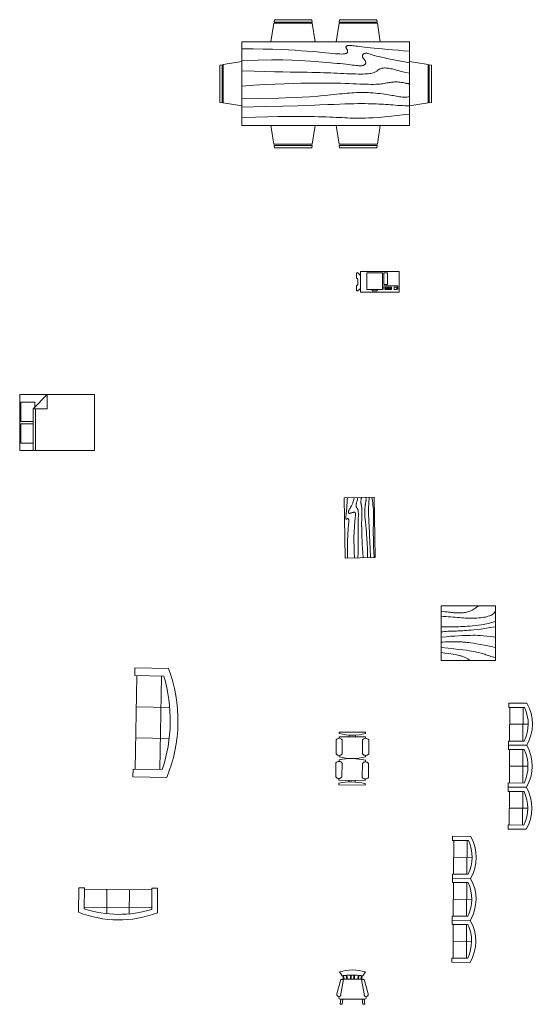
# Model space of a CAD drawing. Units: inches. Extents: x -1085 to 1941, y 1514 to 2348.
# Tile 5 of 9: x -255 to 142, y 1589 to 2348. Entities that reach past the tile are written whole.
import ezdxf

# ---------------------------------------------------------------- set-up
doc = ezdxf.new("R2010")
doc.units = ezdxf.units.IN
doc.layers.add('A-EQPM', color=9, linetype='Continuous', lineweight=18)
doc.layers.add('FOUNITR-URE', color=2, linetype='Continuous', lineweight=18)

# ---------------------------------------------------------------- blocks, each defined once
blk = doc.blocks.new('Bed - Queen')
for p, q in [((0, -80.00003), (0, 0)), ((0, 0), (59.99999, 0)), ((59.99999, 0), (59.99999, -80.00003)), ((7.99999, -1.2), (28.79998, -1.2)), ((7.99999, -14.4), (7.99999, -1.2)), ((28.79998, -1.2), (28.79998, -14.4)), ((31.19999, -1.2), (51.99999, -1.2)), ((31.19999, -14.4), (31.19999, -1.2)), ((51.99999, -1.2), (51.99999, -16.4)), ((0, -14.4), (44.8, -14.4)), ((44.8, -16.8), (0, -16.8)), ((59.99999, -29.6), (44.8, -14.4)), ((44.8, -14.4), (44.8, -29.6)), ((51.99999, -16.4), (46.79936, -16.4)), ((44.8, -29.6), (59.99999, -29.6)), ((59.99999, -80.00003), (0, -80.00003))]:
    blk.add_line(p, q)
blk = doc.blocks.new('Chair - Desk')
for p, q in [((-8.5, 0), (-8.5, -1)), ((-8.5, 0), (8.5, 0)), ((8.5, 0), (8.5, -1)), ((-10.5, -5), (-10.5, -14)), ((-8.5, -3), (-8.5, -4)), ((-8.5, -3), (8.5, -3)), ((-6.5, -14), (-6.5, -5)), ((-2, -3), (-2, -1.9355)), ((2, -1.9576), (2, -3)), ((6.5, -5), (6.5, -14)), ((8.5, -3), (8.5, -4)), ((10.5, -14), (10.5, -5)), ((-8.5, -15), (-8.5, -16)), ((8.5, -15), (8.5, -16))]:
    blk.add_line(p, q)
for centre, radius, start, end in [((-8.5, -6.5), 2.5, 36.8699, 143.1301), ((0, 34.625), 36.625, 256.5803, 283.4197), ((8.5, -6.5), 2.5, 36.8699, 143.1301), ((-8.5, -12.5), 2.5, 216.8699, 323.1301), ((0, 19.625), 36.625, 256.5803, 283.4197), ((8.5, -12.5), 2.5, 216.8699, 323.1301)]:
    blk.add_arc(centre, radius, start, end)
blk = doc.blocks.new('Sofa - Roundback Loveseat 5 ft.')
for p, q in [((-24, -33.99998), (-24, -11.46958)), ((-23.9998, -13.38178), (23.99986, -13.38178)), ((0, -32.44198), (0, -5.99998)), ((24.00004, -33.99998), (24.00004, -11.46958)), ((-24, -32.44198), (24.00004, -32.44198))]:
    blk.add_line(p, q)
for points in [[(-24, -33.99998), (-30, -33.99998), (-30, -7.99998)], [(30.00004, -7.99998), (30.00004, -33.99998), (24.00004, -33.99998)]]:
    blk.add_lwpolyline(points)
for centre, radius, start, end in [((0, -60.24998), 60.24998, 60.13715, 119.8628), ((0, -61.38438), 55.38444, 64.32083, 115.6792)]:
    blk.add_arc(centre, radius, start, end)
blk = doc.blocks.new('Table - Square Woodgrain 42 x 42 in.')
blk.add_line((0, -42), (42, -42))
for points in [[(0, -4), (1.704, -4.2172), (3.2358, -4.4188), (4.615, -4.604), (5.8615, -4.7721), (6.9951, -4.9224), (8.0357, -5.0541), (9.0031, -5.1667), (9.9171, -5.2594), (10.7951, -5.3316), (11.6445, -5.3836), (12.4702, -5.4157), (13.277, -5.4283), (14.0698, -5.4217), (14.8535, -5.3964), (15.6331, -5.3526), (16.4133, -5.2908), (17.1986, -5.2103), (17.9913, -5.1062), (18.793, -4.9727), (19.6056, -4.8038), (20.4307, -4.5937), (21.2701, -4.3365), (22.1256, -4.0262), (22.9989, -3.6571), (23.888, -3.2272), (24.7756, -2.7516), (25.6408, -2.2491), (26.4624, -1.7387), (27.2195, -1.2395), (27.891, -0.7703), (28.456, -0.3501), (28.8934, 0.002)], [(0, -42), (0, 0), (42, 0), (42, -42)], [(0, -8), (1.8203, -8.1001), (3.6741, -8.2149), (5.5411, -8.3408), (7.4011, -8.4741), (9.2339, -8.6112), (11.0193, -8.7484), (12.7371, -8.8821), (14.3671, -9.0086), (15.8954, -9.1246), (17.3337, -9.2278), (18.6997, -9.3159), (20.0116, -9.387), (21.2871, -9.4389), (22.5442, -9.4696), (23.8008, -9.477), (25.0749, -9.459), (26.3791, -9.4137), (27.7049, -9.3403), (29.0383, -9.2382), (30.3655, -9.1068), (31.6728, -8.9455), (32.9461, -8.7535), (34.1717, -8.5304), (35.3358, -8.2756), (36.4268, -7.9863), (37.443, -7.6521), (38.3849, -7.2603), (39.253, -6.7986), (40.048, -6.2542), (40.7705, -5.6147), (41.421, -4.8674), (42, -4)], [(42, -12), (39.1784, -12.8621), (36.4519, -13.5654), (33.8246, -14.1294), (31.3004, -14.5731), (28.8832, -14.9161), (26.577, -15.1775), (24.3858, -15.3768), (22.3136, -15.5332), (20.3622, -15.6632), (18.5254, -15.7718), (16.7947, -15.8612), (15.1618, -15.9338), (13.6183, -15.9916), (12.1558, -16.0369), (10.7659, -16.0718), (9.4403, -16.0987), (8.1703, -16.1191), (6.9461, -16.1325), (5.7577, -16.1377), (4.595, -16.1335), (3.4479, -16.1188), (2.3064, -16.0924), (1.1604, -16.0532), (0, -16)], [(42, -16), (37.6529, -16.7365), (33.8802, -17.329), (30.6179, -17.7961), (27.8015, -18.1561), (25.3668, -18.4275), (23.2497, -18.6288), (21.3859, -18.7785), (19.7111, -18.8949), (18.1693, -18.9939), (16.7375, -19.0795), (15.401, -19.1534), (14.1449, -19.217), (12.9544, -19.2717), (11.8148, -19.3191), (10.7113, -19.3606), (9.6291, -19.3976), (8.5534, -19.4323), (7.47, -19.4689), (6.3643, -19.5122), (5.222, -19.5672), (4.0288, -19.6386), (2.7703, -19.7313), (1.4321, -19.8501), (0, -20)], [(0, -24), (3.9243, -23.6805), (7.4766, -23.4138), (10.6891, -23.1954), (13.5943, -23.0205), (16.2247, -22.8847), (18.6125, -22.7832), (20.7903, -22.7116), (22.7903, -22.6651), (24.6563, -22.642), (26.4764, -22.6507), (28.35, -22.7024), (30.3766, -22.8084), (32.6555, -22.98), (35.2861, -23.2283), (38.3678, -23.5645), (42, -24)], [(42, -32), (37.392, -31.017), (33.4585, -30.2231), (30.1291, -29.5949), (27.3334, -29.109), (25.0009, -28.742), (23.0612, -28.4707), (21.4439, -28.2716), (20.0786, -28.1215), (18.8998, -28.0002), (17.8609, -27.9014), (16.9206, -27.8219), (16.0371, -27.7588), (15.1691, -27.709), (14.2748, -27.6693), (13.3128, -27.6368), (12.2415, -27.6083), (11.0295, -27.5824), (9.6867, -27.5643), (8.233, -27.5608), (6.6884, -27.5787), (5.0728, -27.6248), (3.4062, -27.7058), (1.7086, -27.8286), (0, -28)], [(0, -32), (5.4026, -32.5358), (9.9494, -33.019), (13.7424, -33.4553), (16.8834, -33.8505), (19.4743, -34.2106), (21.6171, -34.5413), (23.4136, -34.8486), (24.9657, -35.1382), (26.3614, -35.4156), (27.6332, -35.6841), (28.7995, -35.9467), (29.8788, -36.2064), (30.8897, -36.4661), (31.8507, -36.7288), (32.7802, -36.9973), (33.6968, -37.2747), (34.6175, -37.5635), (35.5531, -37.8651), (36.5128, -38.1805), (37.506, -38.5108), (38.5421, -38.8568), (39.6302, -39.2197), (40.7797, -39.6004), (42, -40)], [(0, -36), (3.0098, -36.2857), (5.5354, -36.5643), (7.6368, -36.8359), (9.374, -37.1009), (10.807, -37.3597), (11.9957, -37.6126), (13.0002, -37.8599), (13.8804, -38.102), (14.6874, -38.3393), (15.4365, -38.5729), (16.1338, -38.8041), (16.7858, -39.0341), (17.3987, -39.264), (17.9787, -39.4952), (18.5322, -39.7288), (19.0655, -39.9662), (19.5832, -40.2081), (20.0842, -40.4544), (20.5657, -40.7046), (21.0249, -40.9581), (21.459, -41.2144), (21.8653, -41.4731), (22.2409, -41.7335), (22.5831, -41.9951)]]:
    blk.add_lwpolyline(points)
blk = doc.blocks.new('Table - Rectangular Woodgrain 60 x 30 in.')
for p, q in [((0, 0), (0, -30)), ((60, 0), (0, 0)), ((60, -30), (60, 0)), ((0, -30), (60, -30))]:
    blk.add_line(p, q)
for points in [[(0, -2.4), (4.8155, -2.418), (9.0302, -2.4688), (12.709, -2.5477), (15.9167, -2.65), (18.7181, -2.7711), (21.1781, -2.9063), (23.3616, -3.0508), (25.3333, -3.2), (27.1477, -3.3495), (28.8172, -3.4958), (30.3437, -3.636), (31.7291, -3.7667), (32.9756, -3.8849), (34.0849, -3.9875), (35.059, -4.0714), (35.9, -4.1334), (36.6114, -4.1711), (37.2041, -4.1854), (37.6906, -4.1779), (38.0833, -4.15), (38.3948, -4.1034), (38.6375, -4.0396), (38.8239, -3.9602), (38.9666, -3.8667), (39.0764, -3.7608), (39.1573, -3.6448), (39.2116, -3.521), (39.2416, -3.3917), (39.2498, -3.2593), (39.2385, -3.1261), (39.21, -2.9944), (39.1666, -2.8667), (39.111, -2.7447), (39.0468, -2.6281), (38.978, -2.5163), (38.9083, -2.4083), (38.8418, -2.3035), (38.7823, -2.201), (38.7337, -2.1001), (38.7, -2), (38.6844, -1.9003), (38.6875, -1.8021), (38.7094, -1.707), (38.75, -1.6167), (38.8094, -1.5326), (38.8875, -1.4563), (38.9844, -1.3893), (39.1, -1.3333), (39.2351, -1.2896), (39.3937, -1.2583), (39.5804, -1.2396), (39.8, -1.2333), (40.057, -1.2396), (40.3562, -1.2583), (40.7023, -1.2896), (41.1, -1.3333), (41.5547, -1.3895), (42.0755, -1.4573), (42.6721, -1.5361), (43.3542, -1.625), (44.1316, -1.7233), (45.014, -1.8302), (46.0114, -1.9449), (47.1333, -2.0667), (48.3862, -2.1947), (49.7625, -2.3281), (51.2513, -2.4663), (52.8416, -2.6083), (54.5226, -2.7535), (56.2833, -2.9011), (58.1127, -3.0501), (60, -3.2)], [(0, -9.2), (6.5759, -9.0858), (11.9385, -9.0365), (16.2527, -9.0418), (19.6833, -9.0917), (22.3952, -9.1759), (24.5531, -9.2844), (26.322, -9.4069), (27.8666, -9.5333), (29.3241, -9.6553), (30.7203, -9.7719), (32.0532, -9.8837), (33.3208, -9.9917), (34.5213, -10.0965), (35.6526, -10.199), (36.7128, -10.2999), (37.7, -10.4), (38.6129, -10.4996), (39.4531, -10.5969), (40.223, -10.6895), (40.925, -10.775), (41.5613, -10.8512), (42.1344, -10.9156), (42.6465, -10.966), (43.1, -11), (43.4976, -11.0158), (43.8437, -11.0136), (44.143, -10.9942), (44.4, -10.9583), (44.6195, -10.9069), (44.8062, -10.8406), (44.9648, -10.7603), (45.1, -10.6667), (45.2155, -10.5598), (45.3114, -10.4365), (45.3871, -10.2929), (45.4416, -10.125), (45.4743, -9.929), (45.4844, -9.7011), (45.4709, -9.4371), (45.4333, -9.1333), (45.3716, -8.7883), (45.2896, -8.4104), (45.1919, -8.0107), (45.0833, -7.6), (44.9685, -7.1893), (44.8521, -6.7896), (44.7388, -6.4117), (44.6333, -6.0667), (44.54, -5.7628), (44.4614, -5.4979), (44.4001, -5.2675), (44.3583, -5.0667), (44.3384, -4.8909), (44.3427, -4.7354), (44.3736, -4.5956), (44.4333, -4.4667), (44.5236, -4.3453), (44.6427, -4.2333), (44.7884, -4.1339), (44.9583, -4.05), (45.1501, -3.9849), (45.3614, -3.9417), (45.59, -3.9234), (45.8333, -3.9333), (46.0915, -3.9749), (46.3734, -4.0531), (46.6906, -4.1736), (47.0542, -4.3417), (47.4756, -4.5629), (47.9661, -4.8427), (48.5372, -5.1866), (49.2, -5.6), (49.9676, -6.0844), (50.8594, -6.625), (51.8965, -7.2031), (53.1, -7.8), (54.491, -8.3969), (56.0906, -8.975), (57.9199, -9.5156), (60, -10)], [(0, -12.8), (5.1847, -12.9322), (9.6213, -13.0323), (13.3963, -13.1059), (16.5958, -13.1583), (19.3063, -13.1952), (21.614, -13.2219), (23.6054, -13.2439), (25.3666, -13.2667), (26.9728, -13.2947), (28.4531, -13.3281), (29.8256, -13.3663), (31.1083, -13.4083), (32.3191, -13.4535), (33.476, -13.501), (34.597, -13.5501), (35.7, -13.6), (36.7984, -13.6497), (37.8875, -13.6979), (38.9578, -13.743), (40, -13.7833), (41.0047, -13.8174), (41.9625, -13.8438), (42.864, -13.8607), (43.7, -13.8667), (44.4631, -13.8604), (45.1552, -13.8417), (45.7801, -13.8104), (46.3416, -13.7667), (46.8439, -13.7104), (47.2906, -13.6417), (47.6858, -13.5604), (48.0333, -13.4667), (48.3375, -13.3608), (48.6042, -13.2448), (48.8396, -13.121), (49.05, -12.9917), (49.2417, -12.8593), (49.4208, -12.7261), (49.5937, -12.5944), (49.7667, -12.4667), (49.9452, -12.3451), (50.1323, -12.2313), (50.3303, -12.1268), (50.5416, -12.0333), (50.7686, -11.9524), (51.0135, -11.8854), (51.2788, -11.8341), (51.5666, -11.8), (51.8785, -11.7843), (52.2116, -11.7865), (52.562, -11.8059), (52.926, -11.8417), (53.2998, -11.8931), (53.6795, -11.9594), (54.0614, -12.0397), (54.4416, -12.1333), (54.8223, -12.2401), (55.2293, -12.3625), (55.6942, -12.5037), (56.2489, -12.6667), (56.9251, -12.8547), (57.7545, -13.0708), (58.7689, -13.3182), (60, -13.6)], [(0, -18), (5.124, -17.7273), (9.6609, -17.5057), (13.6705, -17.3303), (17.2125, -17.1958), (20.3467, -17.0973), (23.1328, -17.0297), (25.6307, -16.9878), (27.9, -16.9667), (29.9928, -16.9617), (31.9302, -16.9703), (33.7254, -16.9907), (35.3917, -17.0208), (36.9423, -17.0588), (38.3906, -17.1026), (39.7499, -17.1503), (41.0333, -17.2), (42.2519, -17.2496), (43.4073, -17.2969), (44.4986, -17.3395), (45.525, -17.375), (46.4858, -17.4012), (47.3802, -17.4156), (48.2074, -17.416), (48.9667, -17.4), (49.6583, -17.3662), (50.2872, -17.3167), (50.8595, -17.2547), (51.3812, -17.1833), (51.8584, -17.1057), (52.2971, -17.025), (52.7034, -16.9443), (53.0833, -16.8667), (53.443, -16.7951), (53.789, -16.7313), (54.128, -16.6768), (54.4666, -16.6334), (54.8115, -16.6024), (55.1693, -16.5854), (55.5465, -16.5841), (55.95, -16.6), (56.3828, -16.6337), (56.8346, -16.6823), (57.2915, -16.7418), (57.7396, -16.8084), (58.165, -16.878), (58.5539, -16.9469), (58.8924, -17.0111), (59.1666, -17.0667), (59.3679, -17.1107), (59.5078, -17.1438), (59.6032, -17.1675), (59.6708, -17.1833), (59.7275, -17.193), (59.7901, -17.1979), (59.8753, -17.1998), (60, -17.2)], [(0, -22.4), (8.0098, -22.2501), (14.4094, -22.1011), (19.4168, -21.9535), (23.25, -21.8083), (26.1269, -21.6663), (28.2656, -21.5281), (29.884, -21.3947), (31.2, -21.2667), (32.3967, -21.1448), (33.5172, -21.0292), (34.5697, -20.9198), (35.5625, -20.8167), (36.5037, -20.7198), (37.4015, -20.6292), (38.2642, -20.5448), (39.1, -20.4667), (39.9164, -20.3951), (40.7187, -20.3313), (41.5117, -20.2768), (42.3, -20.2333), (43.0883, -20.2024), (43.8812, -20.1854), (44.6836, -20.1841), (45.5, -20.2), (46.3328, -20.234), (47.1747, -20.2844), (48.0163, -20.3488), (48.8479, -20.425), (49.66, -20.5106), (50.4429, -20.6031), (51.1872, -20.7004), (51.8833, -20.8), (52.5246, -20.8999), (53.1166, -20.9995), (53.6681, -21.0983), (54.1875, -21.1958), (54.6834, -21.2919), (55.1646, -21.3859), (55.6394, -21.4777), (56.1167, -21.5667), (56.6028, -21.6515), (57.0961, -21.7266), (57.5929, -21.7852), (58.0896, -21.8208), (58.5823, -21.8268), (59.0674, -21.7964), (59.5412, -21.723), (60, -21.6)], [(0, -25.2), (8.6355, -25.0504), (15.7026, -24.9031), (21.4049, -24.7606), (25.9458, -24.625), (29.529, -24.4988), (32.3578, -24.3844), (34.6359, -24.284), (36.5667, -24.2), (38.3213, -24.1341), (39.9417, -24.0854), (41.437, -24.0523), (42.8167, -24.0333), (44.0901, -24.0268), (45.2667, -24.0313), (46.3557, -24.0451), (47.3667, -24.0667), (48.309, -24.0947), (49.1928, -24.1287), (50.0284, -24.168), (50.826, -24.2125), (51.5959, -24.2617), (52.3483, -24.3151), (53.0935, -24.3725), (53.8417, -24.4334), (54.6009, -24.497), (55.3699, -24.561), (56.1454, -24.6226), (56.9239, -24.6792), (57.7021, -24.7279), (58.4764, -24.7662), (59.2435, -24.7911), (60, -24.8)], [(0, -28.8), (5.6867, -28.6681), (10.45, -28.5698), (14.407, -28.5012), (17.675, -28.4584), (20.3711, -28.4374), (22.6125, -28.4344), (24.5164, -28.4455), (26.2, -28.4667), (27.762, -28.4947), (29.2276, -28.5281), (30.6033, -28.5663), (31.8958, -28.6084), (33.1118, -28.6535), (34.2578, -28.7011), (35.3405, -28.7501), (36.3666, -28.8), (37.3443, -28.8497), (38.288, -28.8974), (39.2137, -28.9412), (40.1375, -28.9792), (41.0753, -29.0093), (42.0432, -29.0297), (43.0572, -29.0384), (44.1333, -29.0333), (45.2936, -29.0114), (46.5843, -28.9641), (48.0579, -28.8816), (49.7666, -28.7542), (51.7629, -28.5721), (54.0989, -28.3255), (56.8272, -28.0048), (60, -27.6)]]:
    blk.add_lwpolyline(points)
blk = doc.blocks.new('Copy Machine')
for p, q in [((0, 0), (0, -16)), ((30, 0), (0, 0)), ((30, -16), (30, 0)), ((-3, -1), (-3, -5)), ((-2, -1), (-3, -1)), ((-3, -5), (-2, -6)), ((0, -3), (-2, -1)), ((-2, -10), (-2, -6)), ((5, -1), (5, -14)), ((17, -1), (5, -1)), ((17, -14), (17, -1)), ((18, -1), (18, -10)), ((21, -1), (18, -1)), ((21, -10), (21, -1)), ((-3, -11), (-2, -10)), ((-3, -15), (-3, -11)), ((-2, -15), (-3, -15)), ((0, -13), (-2, -15)), ((5, -14), (17, -14)), ((9, -14), (9, -15)), ((9, -15), (13, -15)), ((13, -15), (13, -14)), ((18, -10), (21, -10)), ((18, -14), (18, -11)), ((18, -11), (29, -11)), ((24, -12), (19, -12)), ((19, -12), (19, -14)), ((24, -13), (19, -13)), ((19, -14), (24, -14)), ((20, -12), (20, -14)), ((21, -14), (21, -12)), ((22, -12), (22, -14)), ((23, -14), (23, -12)), ((24, -14), (24, -12)), ((28, -12), (26, -12)), ((26, -12), (26, -14)), ((26, -14), (28, -14)), ((28, -14), (28, -12)), ((29, -11), (29, -14)), ((0, -16), (30, -16))]:
    blk.add_line(p, q)
blk = doc.blocks.new('Chair - Rocking')
for p, q in [((-9, -7.5), (-12, -18.49999)), ((-8, -4.5), (-10, -1.5)), ((-7, -7.5), (-9, -7.5)), ((-9, -18.49999), (-7, -7.5)), ((-8.23428, -6.99939), (-8.3093, -7.47958)), ((-8.23041, -7), (8.23915, -7)), ((-7.5, -4.5), (-7, -7)), ((-6.5, -7), (-7.02225, -4.43)), ((-4.5, -7), (-4.96674, -4.19951)), ((-4, -7), (-4.40532, -4.16272)), ((-1.5, -4.05012), (-1.5, -7)), ((-1, -7), (-1, -4.05012)), ((1, -7), (1, -4.04655)), ((1.5, -4.05012), (1.5, -7)), ((4, -7), (4.40187, -4.18694)), ((4.5, -7), (4.96761, -4.19437)), ((6.5, -7), (7, -4.4057)), ((7.5, -4.5), (7, -7)), ((7, -7.5), (9, -7.5)), ((9, -18.49999), (7, -7.5)), ((8, -4.5), (10, -1.5)), ((8.31071, -7.48854), (8.23449, -7.00073)), ((9, -7.5), (12, -18.49999)), ((-10.36644, -20.64523), (-10.5, -21.49999)), ((-9, -22.49999), (-9.5, -26.49999)), ((0, -22.49999), (-9.5, -22.49999)), ((-8, -26.49999), (-7.5, -22.49999)), ((0, -22.49999), (9.5, -22.49999)), ((8, -26.49999), (7.5, -22.49999)), ((9, -22.49999), (9.5, -26.49999)), ((10.5, -21.49999), (10.3575, -20.58798)), ((-9.5, -26.49999), (-8, -26.49999)), ((9.5, -26.49999), (8, -26.49999))]:
    blk.add_line(p, q)
for centre, radius, start, end in [((0, -34.08333), 34.08333, 72.93847, 107.0615), ((0, -68.25004), 64.25, 93.92211, 97.15267), ((0, -68.25004), 64.25, 82.84733, 93.92211), ((-10.5, -18.99999), 1.58114, 161.5651, 18.43495), ((-9.5, -21.49999), 1, 180, 270), ((10.5, -18.99999), 1.58114, 161.5651, 18.43495), ((9.5, -21.49999), 1, 270, 0)]:
    blk.add_arc(centre, radius, start, end)
blk = doc.blocks.new('Dining Set - 36 x 72 in.')
for p, q in [((-22.2343, 26.00059), (-23.4847, 17.99762)), ((-22.2304, 26), (-5.7608, 26)), ((-22, 27.5), (-22.1562, 26.50042)), ((-5.8416, 26.5), (-22.1534, 26.5)), ((-22, 27.5), (-6, 27.5)), ((-5.8437, 26.49966), (-6, 27.5)), ((-4.5152, 17.99762), (-5.7655, 25.99926)), ((5.7657, 26.00059), (4.5153, 17.99762)), ((5.7696, 26), (22.2392, 26)), ((6, 27.5), (5.8438, 26.50042)), ((22.1584, 26.5), (5.8466, 26.5)), ((6, 27.5), (22, 27.5)), ((22.1563, 26.49966), (22, 27.5)), ((23.4848, 17.99762), (22.2345, 25.99926)), ((36, 18), (-36, 18)), ((-36, 18), (-36, -18)), ((36, -18), (36, 18)), ((-44.0006, 8.23428), (-35.9976, 9.48474)), ((44.0006, 8.23428), (35.9976, 9.48474)), ((-45.5, 8), (-44.5004, 8.15617)), ((-45.5, 8), (-45.5, -8)), ((-44.5, -8.15843), (-44.5, 8.15338)), ((-44, 8.23041), (-44, -8.23915)), ((44, 8.23041), (44, -8.23915)), ((44.5, -8.15843), (44.5, 8.15338)), ((45.5, 8), (44.5005, 8.15617)), ((45.5, 8), (45.5, -8)), ((-44.4997, -8.15631), (-45.5, -8)), ((-35.9976, -9.48476), (-43.9993, -8.2345)), ((35.9976, -9.48476), (43.9993, -8.2345)), ((44.4997, -8.15631), (45.5, -8)), ((-36, -18), (36, -18)), ((-22.2343, -26.0006), (-23.4847, -17.99762)), ((-4.5152, -17.99762), (-5.7655, -25.99928)), ((5.7657, -26.0006), (4.5153, -17.99762)), ((23.4848, -17.99762), (22.2345, -25.99928)), ((-22.2304, -26), (-5.7608, -26)), ((-22, -27.5), (-22.1562, -26.50044)), ((-5.8416, -26.5), (-22.1534, -26.5)), ((-22, -27.5), (-6, -27.5)), ((-5.8437, -26.49967), (-6, -27.5)), ((5.7696, -26), (22.2392, -26)), ((6, -27.5), (5.8438, -26.50044)), ((22.1584, -26.5), (5.8466, -26.5)), ((6, -27.5), (22, -27.5)), ((22.1563, -26.49967), (22, -27.5))]:
    blk.add_line(p, q)
for points in [[(-36, 15), (-31.1772, 14.97754), (-26.8079, 14.91406), (-22.8538, 14.81543), (-19.276, 14.6875), (-16.0362, 14.53613), (-13.0957, 14.36718), (-10.4159, 14.18652), (-7.9583, 14), (-5.6904, 13.81315), (-3.6035, 13.63021), (-1.6954, 13.45508), (0.0365, 13.29166), (1.5945, 13.14388), (2.9811, 13.01562), (4.1988, 12.9108), (5.25, 12.83333), (6.1393, 12.78613), (6.8802, 12.76823), (7.4883, 12.77767), (7.9792, 12.8125), (8.3685, 12.87077), (8.6719, 12.95052), (8.9049, 13.0498), (9.0833, 13.16666), (9.2205, 13.29899), (9.3216, 13.44401), (9.3895, 13.59879), (9.4271, 13.76041), (9.4373, 13.92594), (9.4232, 14.09245), (9.3875, 14.257), (9.3333, 14.41666), (9.2638, 14.56917), (9.1836, 14.71484), (9.0975, 14.85465), (9.0104, 14.98958), (8.9272, 15.1206), (8.8529, 15.2487), (8.7922, 15.37483), (8.75, 15.5), (8.7305, 15.62467), (8.7344, 15.74739), (8.7617, 15.86621), (8.8125, 15.97916), (8.8867, 16.08431), (8.9844, 16.17968), (9.1055, 16.26334), (9.25, 16.33333), (9.4189, 16.38802), (9.6172, 16.42708), (9.8506, 16.45052), (10.125, 16.45833), (10.4463, 16.45052), (10.8203, 16.42708), (11.2529, 16.38802), (11.75, 16.33333), (12.3184, 16.26318), (12.9694, 16.17838), (13.7151, 16.07991), (14.5677, 15.96875), (15.5395, 15.84586), (16.6426, 15.71224), (17.8893, 15.56884), (19.2917, 15.41666), (20.859, 15.25667), (22.5879, 15.08984), (24.4721, 14.91715), (26.5052, 14.73958), (28.6809, 14.5581), (30.9929, 14.3737), (33.4347, 14.18733), (36, 14)], [(-36, 10), (-28.9766, 10.14274), (-23.1725, 10.20442), (-18.4241, 10.19775), (-14.5677, 10.13541), (-11.4399, 10.03011), (-8.877, 9.89453), (-6.7154, 9.74137), (-4.7917, 9.58333), (-2.9698, 9.43082), (-1.2246, 9.28515), (0.4415, 9.14534), (2.026, 9.01041), (3.5266, 8.87939), (4.9408, 8.7513), (6.266, 8.62516), (7.5, 8.5), (8.6411, 8.37549), (9.6914, 8.2539), (10.6538, 8.13818), (11.5312, 8.03125), (12.3267, 7.93603), (13.043, 7.85547), (13.6831, 7.79248), (14.25, 7.75), (14.7471, 7.7303), (15.1797, 7.73307), (15.5537, 7.75732), (15.875, 7.80208), (16.1494, 7.86637), (16.3828, 7.94922), (16.5811, 8.04964), (16.75, 8.16666), (16.8944, 8.29915), (17.0143, 8.44531), (17.1089, 8.60319), (17.1771, 8.77083), (17.218, 8.94629), (17.2305, 9.1276), (17.2137, 9.31282), (17.1667, 9.5), (17.0895, 9.6875), (16.987, 9.875), (16.8649, 10.0625), (16.7292, 10.25), (16.5856, 10.4375), (16.4401, 10.625), (16.2985, 10.8125), (16.1667, 11), (16.05, 11.18733), (15.9518, 11.3737), (15.8752, 11.5581), (15.8229, 11.73958), (15.798, 11.91715), (15.8034, 12.08984), (15.842, 12.25667), (15.9167, 12.41666), (16.0295, 12.56836), (16.1784, 12.70833), (16.3605, 12.83268), (16.5729, 12.9375), (16.8127, 13.01888), (17.0768, 13.07291), (17.3625, 13.0957), (17.6667, 13.08333), (17.9894, 13.03312), (18.3418, 12.94726), (18.7382, 12.82918), (19.1927, 12.68229), (19.7195, 12.51001), (20.3327, 12.31575), (21.0465, 12.10294), (21.875, 11.875), (22.8357, 11.63354), (23.959, 11.37304), (25.2786, 11.08618), (26.8282, 10.76562), (28.6414, 10.40405), (30.752, 9.99414), (33.1936, 9.52856), (36, 9)], [(-36, 5.5), (-30.7157, 5.3348), (-26.069, 5.20963), (-21.9946, 5.11767), (-18.4271, 5.05208), (-15.3009, 5.00602), (-12.5508, 4.97265), (-10.1112, 4.94515), (-7.9167, 4.91666), (-5.909, 4.88167), (-4.0586, 4.83984), (-2.3429, 4.79215), (-0.7396, 4.73958), (0.7739, 4.6831), (2.22, 4.6237), (3.6213, 4.56233), (5, 4.5), (6.373, 4.43782), (7.7344, 4.3776), (9.0723, 4.32129), (10.375, 4.27083), (11.6309, 4.22819), (12.8281, 4.19531), (13.9551, 4.17415), (15, 4.16666), (15.954, 4.17448), (16.819, 4.19791), (17.6001, 4.23698), (18.3021, 4.29166), (18.9299, 4.36198), (19.4883, 4.44791), (19.9823, 4.54948), (20.4167, 4.66666), (20.7969, 4.79899), (21.1302, 4.94401), (21.4245, 5.09879), (21.6875, 5.26041), (21.9271, 5.42594), (22.1511, 5.59245), (22.3672, 5.757), (22.5834, 5.91666), (22.8065, 6.06868), (23.0404, 6.21093), (23.2879, 6.34147), (23.5521, 6.45833), (23.8358, 6.55957), (24.142, 6.64323), (24.4735, 6.70735), (24.8334, 6.75), (25.2235, 6.76969), (25.642, 6.76692), (26.0858, 6.74267), (26.5521, 6.69791), (27.0379, 6.63362), (27.5404, 6.55078), (28.0565, 6.45036), (28.5834, 6.33333), (29.1242, 6.19987), (29.7071, 6.04687), (30.3661, 5.87044), (31.1354, 5.66666), (32.0493, 5.43164), (33.142, 5.16146), (34.4475, 4.85221), (36, 4.5)], [(-36, -1), (-30.7915, -0.6591), (-26.0195, -0.38216), (-21.6519, -0.16284), (-17.6563, 0.00521), (-14.0005, 0.12833), (-10.6523, 0.21289), (-7.5796, 0.26522), (-4.75, 0.29166), (-2.134, 0.29793), (0.2878, 0.28711), (2.5317, 0.26163), (4.6146, 0.22396), (6.5529, 0.17651), (8.3633, 0.12174), (10.0623, 0.06209), (11.6667, 0), (13.1899, -0.06201), (14.6341, -0.1211), (15.9982, -0.17432), (17.2813, -0.21875), (18.4823, -0.25147), (19.6003, -0.26953), (20.6343, -0.27002), (21.5834, -0.25), (22.4481, -0.20768), (23.2357, -0.14584), (23.9549, -0.06836), (24.6146, 0.02083), (25.2235, 0.11784), (25.7904, 0.21875), (26.3241, 0.31966), (26.8334, 0.41666), (27.3265, 0.50618), (27.8099, 0.58593), (28.2894, 0.65397), (28.7709, 0.70833), (29.2601, 0.74707), (29.763, 0.76823), (30.2855, 0.76985), (30.8334, 0.75), (31.4088, 0.70784), (31.9994, 0.64713), (32.589, 0.57275), (33.1615, 0.48958), (33.7008, 0.4025), (34.1908, 0.3164), (34.6153, 0.23616), (34.9584, 0.16666), (35.2099, 0.11165), (35.3848, 0.07031), (35.504, 0.04069), (35.5886, 0.02083), (35.6594, 0.00879), (35.7377, 0.0026), (35.8442, 0.00032), (36, 0)], [(-36, -6.5), (-27.1843, -6.31267), (-20.084, -6.1263), (-14.469, -5.9419), (-10.1094, -5.76042), (-6.7752, -5.58285), (-4.2363, -5.41016), (-2.2629, -5.24333), (-0.625, -5.08334), (0.8708, -4.93099), (2.2715, -4.78646), (3.5872, -4.64974), (4.8281, -4.52084), (6.0046, -4.39974), (7.127, -4.28646), (8.2053, -4.18099), (9.25, -4.08334), (10.2705, -3.99382), (11.2734, -3.91407), (12.2647, -3.84603), (13.25, -3.79167), (14.2354, -3.75293), (15.2266, -3.73177), (16.2295, -3.73015), (17.25, -3.75), (18.2912, -3.79248), (19.3451, -3.85547), (20.4009, -3.93604), (21.4479, -4.03125), (22.4754, -4.13819), (23.4727, -4.25391), (24.4289, -4.37549), (25.3334, -4.5), (26.1785, -4.62492), (26.9694, -4.74935), (27.7145, -4.87281), (28.4219, -4.99479), (29.1, -5.11483), (29.7572, -5.23242), (30.4016, -5.34709), (31.0417, -5.45834), (31.6837, -5.56437), (32.3262, -5.65821), (32.9658, -5.73153), (33.599, -5.77604), (34.2224, -5.78345), (34.8327, -5.74545), (35.4264, -5.65373), (36, -5.5)], [(-36, -10), (-26.4022, -9.81299), (-18.4675, -9.62891), (-11.9839, -9.45069), (-6.7396, -9.28125), (-2.5226, -9.12354), (0.8789, -8.98047), (3.6769, -8.85498), (6.0833, -8.75), (8.2767, -8.66765), (10.3021, -8.60677), (12.1712, -8.56543), (13.8958, -8.54167), (15.4876, -8.53353), (16.9583, -8.53907), (18.3197, -8.55632), (19.5834, -8.58334), (20.7616, -8.61841), (21.8685, -8.66081), (22.9188, -8.71004), (23.9271, -8.76563), (24.9081, -8.82707), (25.8763, -8.89388), (26.8465, -8.96558), (27.8334, -9.04167), (28.8474, -9.12118), (29.8828, -9.20117), (30.93, -9.27824), (31.9792, -9.34896), (33.0205, -9.40991), (34.0443, -9.45768), (35.0407, -9.48885), (36, -9.5)], [(-36, -14.5), (-30.0881, -14.33513), (-25.0332, -14.21224), (-20.7312, -14.12647), (-17.0781, -14.07292), (-13.97, -14.04671), (-11.3027, -14.04297), (-8.9724, -14.05681), (-6.875, -14.08334), (-4.9224, -14.11833), (-3.0905, -14.16016), (-1.3709, -14.20785), (0.2448, -14.26042), (1.7647, -14.3169), (3.1973, -14.3763), (4.5507, -14.43767), (5.8333, -14.5), (7.0554, -14.5621), (8.235, -14.62175), (9.3922, -14.67652), (10.5469, -14.72396), (11.7192, -14.76164), (12.929, -14.78711), (14.1965, -14.79794), (15.5417, -14.79167), (16.9933, -14.76424), (18.6152, -14.70508), (20.4804, -14.60197), (22.6615, -14.44271), (25.2312, -14.21509), (28.2624, -13.9069), (31.8277, -13.50594), (36, -13)]]:
    blk.add_lwpolyline(points)
blk = doc.blocks.new('Sofa - Roundback 7 ft.')
for p, q in [((-12.00002, -32.4421), (-12.00003, -6.5971)), ((11.99997, -32.4421), (11.99998, -6.5971)), ((-36.000027, -34), (-36.000027, -11.4696)), ((-35.999844, -13.3819), (35.9998, -13.3819)), ((35.99998, -34), (35.99998, -11.4696)), ((-36.000027, -32.4421), (35.99998, -32.4421))]:
    blk.add_line(p, q)
for points in [[(-36.000027, -34), (-42.000027, -34), (-42.000027, -8)], [(41.99998, -8), (41.99998, -34), (35.99998, -34)]]:
    blk.add_lwpolyline(points)
for centre, radius, start, end in [((0, -114.25), 114.25, 68.43141, 111.5686), ((-0.00001, -127.1968), 121.1968, 72.72033, 107.2797)]:
    blk.add_arc(centre, radius, start, end)

msp = doc.modelspace()

# ---------------------------------------------------------------- block references
at = {"layer": 'A-EQPM'}
msp.add_blockref('Copy Machine', (8.1286, 2153.685), dxfattribs=at)
at = {"layer": 'FOUNITR-URE'}
for name, p, xscale, yscale, zscale in [('Dining Set - 36 x 72 in.', (-18.6725, 2298.3579), 1.7948577999818, 1.7948577999818, 1.7948577999818), ('Chair - Desk', (1.9414, 1798.7046), 1.198560681527003, 1.198560681527003, 1.198560681527003)]:
    msp.add_blockref(name, p, dxfattribs=dict(at, xscale=xscale, yscale=yscale, zscale=zscale))
for name, p, xscale, yscale, zscale, rotation in [('Bed - Queen', (-254.6714, 2015.6015), 0.7204725837382432, 0.7204725837382432, 0.7204725837382432, 90.01605390430686), ('Table - Rectangular Woodgrain 60 x 30 in.', (-3.6361, 1932.8439), 0.7739415990810241, 0.7739415990810241, 0.7739415990810241, 90.90402502805208), ('Sofa - Roundback Loveseat 5 ft.', (140.8207, 1804.6714), 0.5391437841071741, 0.5391437841071741, 0.5391437841071741, 269.6684342890045), ('Sofa - Roundback Loveseat 5 ft.', (140.6334, 1772.3233), 0.5391437841071741, 0.5391437841071741, 0.5391437841071741, 269.6684342890045), ('Chair - Desk', (1.5793, 1757.9567), -1.198560681527003, 1.198560681527003, 1.198560681527003, 178.9819179435781), ('Sofa - Roundback Loveseat 5 ft.', (140.4462, 1739.9752), 0.5391437841071741, 0.5391437841071741, 0.5391437841071741, 269.6684342890045), ('Sofa - Roundback Loveseat 5 ft.', (97.5163, 1702.1122), 0.5391437841071741, 0.5391437841071741, 0.5391437841071741, 269.6684342890045), ('Sofa - Roundback Loveseat 5 ft.', (97.329, 1669.7641), 0.5391437841071741, 0.5391437841071741, 0.5391437841071741, 269.6684342890045), ('Sofa - Roundback 7 ft.', (-178.8629, 1653.9005), 0.7237795177670652, 0.7237795177670652, 0.7237795177670652, 179.6235229613476), ('Sofa - Roundback Loveseat 5 ft.', (97.1418, 1637.416), 0.5391437841071741, 0.5391437841071741, 0.5391437841071741, 269.6684342890045)]:
    msp.add_blockref(name, p, dxfattribs=dict(at, xscale=xscale, yscale=yscale, zscale=zscale, rotation=rotation))
for name, p in [('Table - Square Woodgrain 42 x 42 in.', (70.3323, 1895.9265)), ('Chair - Rocking', (2.06, 1615.4246))]:
    msp.add_blockref(name, p, dxfattribs=at)
at = {"layer": 'FOUNITR-URE', "rotation": 269.0061411650281}
msp.add_blockref('Sofa - Roundback 7 ft.', (-132.5629, 1805.6312), dxfattribs=at)

doc.saveas('drawing.dxf')
